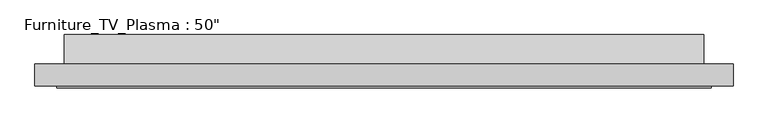
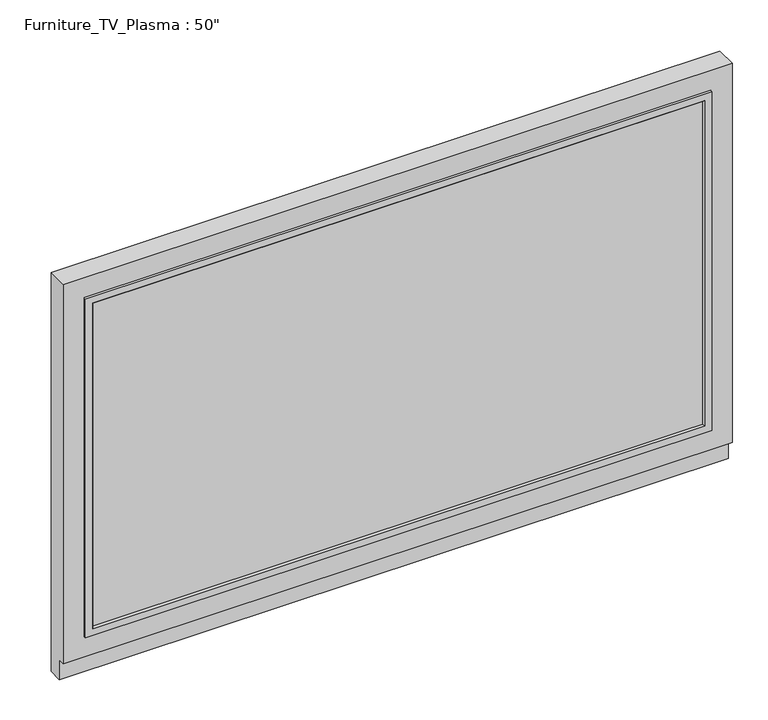
"""IFC4 building model written with IfcOpenShell, lengths in millimetres: furniture geometry."""

from ifc_helpers import new_model, si_unit, frame, origin, place, context, project, spatial, polyline, outline, extrude, faceted_brep, source, transform, mapped, element, save


def furniture_eb486d47(model_context):
    return source(origin(), model_context, "Body", "SolidModel", [
        faceted_brep([(660.4, -50.8, 762.0), (-546.1, -50.8, 762.0), (-546.1, -88.9, 762.0), (660.4, -88.9, 762.0), (-546.1, -50.8, 0.0), (660.4, -50.8, 0.0), (660.4, -76.2, 0.0), (-546.1, -76.2, 0.0), (-546.1, -76.2, 38.1), (-546.1, -88.9, 38.1), (660.4, -88.9, 38.1), (622.3, -88.9, 723.9), (622.3, -88.9, 76.2), (-508.0, -88.9, 76.2), (-508.0, -88.9, 723.9), (660.4, -76.2, 38.1), (622.3, -74.1720413, 723.9), (-508.0, -74.1720413, 723.9), (-508.0, -74.1720413, 76.2), (622.3, -74.1720413, 76.2)], [[[0, 1, 2, 3]], [[4, 5, 6, 7]], [[1, 0, 5, 4]], [[2, 1, 4, 7, 8, 9]], [[3, 2, 9, 10], [11, 12, 13, 14]], [[0, 3, 10, 15, 6, 5]], [[16, 17, 18, 19]], [[16, 19, 12, 11]], [[19, 18, 13, 12]], [[18, 17, 14, 13]], [[17, 16, 11, 14]], [[15, 8, 7, 6]], [[8, 15, 10, 9]]]),
        extrude(outline(polyline([(609.6, -88.9), (-495.3, -88.9), (-495.3, -74.1720413), (609.6, -74.1720413), (609.6, -88.9)])), frame((0.0, 0.0, 88.9), z_axis=(0.0, 0.0, 1.0), x_axis=(1.0, 0.0, 0.0)), (0.0, 0.0, 1.0), 622.3),
        extrude(outline(polyline([(0.0, 676.4688953), (0.0, 38.1), (-50.8, 38.1), (-50.8, 711.2), (0.0, 676.4688953)])), frame((-495.3, 0.0, 0.0), z_axis=(1.0, 0.0, 0.0), x_axis=(0.0, 1.0, 0.0)), (0.0, 0.0, 1.0), 1104.9),
        faceted_brep([(606.425, -88.9, 92.075), (609.6, -92.075, 88.9), (609.6, -92.075, 710.40625), (606.425, -88.9, 707.23125), (609.6, -74.1720413, 88.9), (609.6, -88.9, 88.9), (609.6, -88.9, 710.40625), (609.6, -74.1720413, 710.40625), (622.3, -92.075, 76.2), (622.3, -74.1720413, 76.2), (622.3, -74.1720413, 723.10625), (622.3, -92.075, 723.10625), (-495.3, -92.075, 710.40625), (-492.125, -88.9, 707.23125), (-495.3, -88.9, 710.40625), (-495.3, -74.1720413, 710.40625), (-508.0, -74.1720413, 723.10625), (-508.0, -92.075, 723.10625), (-495.3, -92.075, 88.9), (-492.125, -88.9, 92.075), (-495.3, -88.9, 88.9), (-495.3, -74.1720413, 88.9), (-508.0, -74.1720413, 76.2), (-508.0, -92.075, 76.2)], [[[0, 1, 2, 3]], [[4, 5, 6, 7]], [[8, 9, 10, 11]], [[3, 2, 12, 13]], [[7, 6, 14, 15]], [[11, 10, 16, 17]], [[13, 12, 18, 19]], [[15, 14, 20, 21]], [[17, 16, 22, 23]], [[11, 17, 23, 8], [1, 18, 12, 2]], [[19, 18, 1, 0]], [[5, 20, 14, 6], [3, 13, 19, 0]], [[21, 20, 5, 4]], [[9, 22, 16, 10], [7, 15, 21, 4]], [[23, 22, 9, 8]]]),
    ])


if __name__ == "__main__":
    model = new_model("IFC4")
    model_context = context("Model", 3, world=origin())
    ifc_project = project(units=[si_unit("LENGTHUNIT", "METRE", prefix="MILLI")], contexts=[model_context])
    site = spatial("IfcSite", under=ifc_project)
    building = spatial("IfcBuilding", under=site)
    placement = place(None, origin())
    furniture_shape = furniture_eb486d47(model_context)
    element("IfcFurniture", 1, ObjectType="Furniture_TV_Plasma : 50\"", at=placement, inside=building, context=model_context, shape_type="MappedRepresentation", body=[
        mapped(furniture_shape, transform((0.0, 0.0, 0.0), x_axis=(1.0, 0.0, 0.0), y_axis=(0.0, 1.0, 0.0), z_axis=(0.0, 0.0, 1.0))),
    ])
    save(model, "model.ifc")

# Revit data of these elements
# Type "Furniture_TV_Plasma : 50\""
#   Keynote = "N"
#   Assembly Code = "E2020200"
#   Depth = 0.291667 ft
#   Height = 2.5 ft
#   Width = 3.958333 ft
#   Material Cabinet = Plastic - Gray
#   Default Elevation = 0
# Element 1 (IfcFurniture, "Furniture_TV_Plasma : 50\"")
#   Materials on its faces: "Plastic - Black", "Plastic - Gray", "Glass"
# Materials
#   "Plastic - Gray": class "Plastic", colour RGB 134 134 134, transparency 0
#   "Plastic - Black": colour RGB 0 0 0, transparency 0
#   "Glass": class "Glass", colour RGB 0 128 192, transparency 0.9, Description = "Soda Lime Glass", Cost = 0
